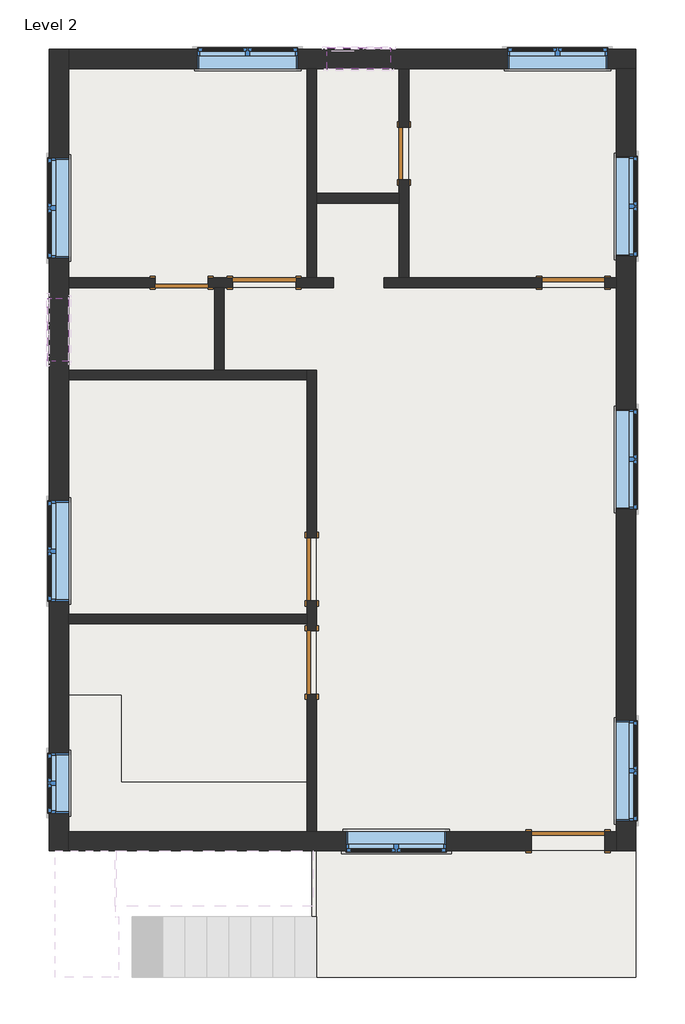
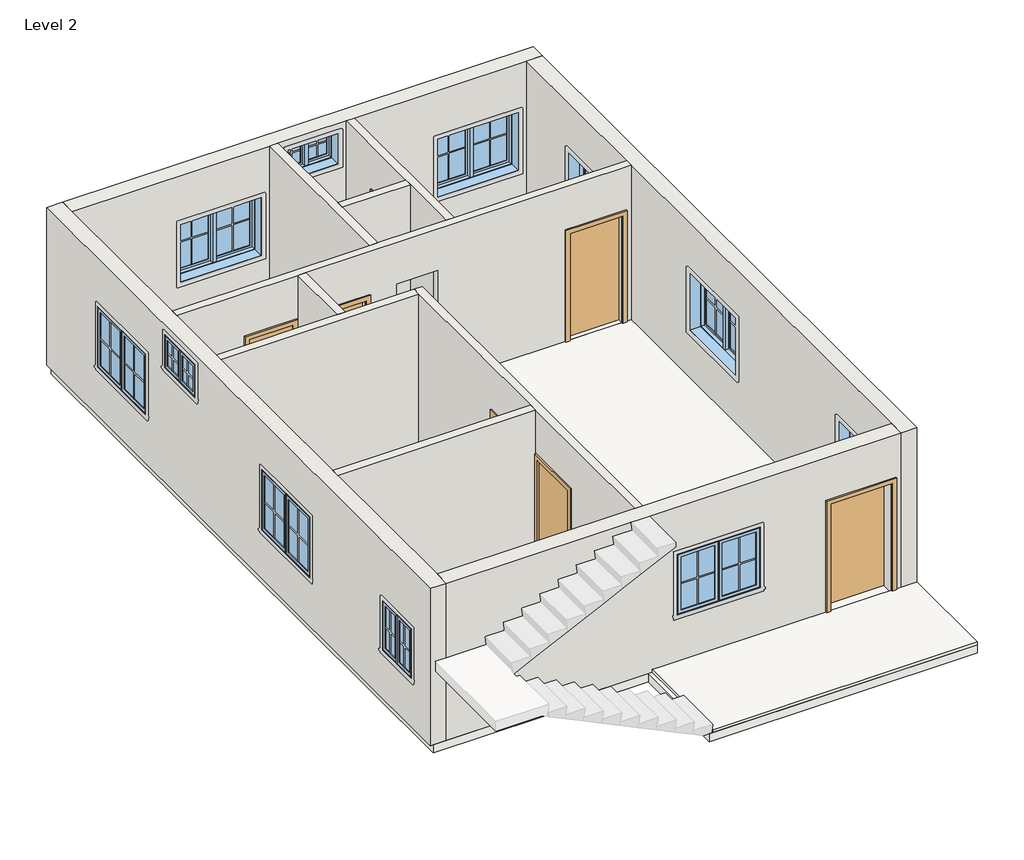
# One storey, part 1 of 2: 12 walls, 11 windows, 7 doors, 6 slabs.
"""IFC4 building model written with IfcOpenShell, lengths in millimetres."""

from ifc_helpers import new_model, si_unit, frame, origin, place, context, project, spatial, polyline, outline, extrude, faceted_brep, transform, mapped, element, save
from components import single_flush_3_6_472124c4, door_c78455d5, door_ad1ac78c, door_798417c2, window_casement_double_3_v2_9f1923e6, window_6eb120d7, window_2333f571

model = new_model("IFC4")

# Units and contexts
model_context = context("Model", 3, world=origin())
ifc_project = project(units=[si_unit("LENGTHUNIT", "METRE", prefix="MILLI")], contexts=[model_context])

# Site, building, storey
site = spatial("IfcSite", under=ifc_project)
building = spatial("IfcBuilding", under=site)
storey = spatial("IfcBuildingStorey", under=building, Name="Level 2", Elevation=3048.0)

# Doors
placement = place(None, origin())
single_flush_3_6_shape = single_flush_3_6_472124c4(model_context)
element("IfcDoor", 1, ObjectType="Single-Flush : 3'6", at=placement, inside=storey, context=model_context, shape_type="MappedRepresentation", body=[
    mapped(single_flush_3_6_shape, transform((-1353.6785282, -4927.3203663, 3048.0), x_axis=(1.0, 0.0, 0.0), y_axis=(0.0, 1.0, 0.0), z_axis=(0.0, 0.0, 1.0))),
])
door_shape = door_c78455d5(model_context)
element("IfcDoor", 2, ObjectType="Single-Flush : 30\" x 80\"", at=placement, inside=storey, context=model_context, shape_type="MappedRepresentation", body=[
    mapped(door_shape, transform((-6936.6570389, 3131.9303819, 3048.0), x_axis=(1.0, 0.0, 0.0), y_axis=(0.0, 1.0, 0.0), z_axis=(0.0, 0.0, 1.0))),
])
element("IfcDoor", 3, ObjectType="Single-Flush : 30\" x 80\"", at=placement, inside=storey, context=model_context, shape_type="MappedRepresentation", body=[
    mapped(door_shape, transform((-3724.1740631, 4999.2141951, 3048.0), x_axis=(0.0, -1.0, 0.0), y_axis=(1.0, 0.0, 0.0), z_axis=(0.0, 0.0, 1.0))),
])
door_2_shape = door_ad1ac78c(model_context)
element("IfcDoor", 4, ObjectType="Single-Flush : 36\" x 80\"", at=placement, inside=storey, context=model_context, shape_type="MappedRepresentation", body=[
    mapped(door_2_shape, transform((-5742.8570389, 3131.9303819, 3048.0), x_axis=(1.0, 0.0, 0.0), y_axis=(0.0, 1.0, 0.0), z_axis=(0.0, 0.0, 1.0))),
])
element("IfcDoor", 5, ObjectType="Single-Flush : 36\" x 80\"", at=placement, inside=storey, context=model_context, shape_type="MappedRepresentation", body=[
    mapped(door_2_shape, transform((-1277.4785282, 3131.9303819, 3048.0), x_axis=(1.0, 0.0, 0.0), y_axis=(0.0, 1.0, 0.0), z_axis=(0.0, 0.0, 1.0))),
])
element("IfcDoor", 6, ObjectType="Single-Flush : 36\" x 80\"", at=placement, inside=storey, context=model_context, shape_type="MappedRepresentation", body=[
    mapped(door_2_shape, transform((-5055.0449828, -2348.5368209, 3048.0), x_axis=(0.0, 1.0, 0.0), y_axis=(-1.0, 0.0, 0.0), z_axis=(0.0, 0.0, 1.0))),
])
door_3_shape = door_798417c2(model_context)
element("IfcDoor", 7, ObjectType="Single-Flush : 36\" x 80\"", at=placement, inside=storey, context=model_context, shape_type="MappedRepresentation", body=[
    mapped(door_3_shape, transform((-5055.0449828, -1002.3368209, 3048.0), x_axis=(0.0, -1.0, 0.0), y_axis=(1.0, 0.0, 0.0), z_axis=(0.0, 0.0, 1.0))),
])

# Slabs
element("IfcSlab", 8, ObjectType="6\"", at=placement, inside=storey, context=model_context, shape_type="SweptSolid", body=[
    extrude(outline(polyline([(-375.7785282, 6451.8796337), (-375.7785282, -6894.0922127), (-5049.0296925, -6894.0922127), (-5049.0296925, -5067.0203663), (-8797.003757, -5067.0203663), (-8797.003757, 6451.8796337), (-375.7785282, 6451.8796337)])), frame((0.0, 0.0, 2895.6), z_axis=(0.0, 0.0, 1.0), x_axis=(1.0, 0.0, 0.0)), (0.0, 0.0, 1.0), 152.4),
])
element("IfcSlab", 9, ObjectType="BED ROOM FLOOR", at=placement, inside=storey, context=model_context, shape_type="SweptSolid", body=[
    extrude(outline(polyline([(-4985.1949828, -4787.6203663), (-8569.7884077, -4787.6203663), (-8569.7884077, -1788.4748314), (-4985.1949828, -1788.4748314), (-4985.1949828, -4787.6203663)])), frame((0.0, 0.0, 3048.0), z_axis=(0.0, 0.0, 1.0), x_axis=(1.0, 0.0, 0.0)), (0.0, 0.0, 1.0), 50.8),
    extrude(outline(polyline([(-4985.1949828, -1672.5465885), (-8569.7884077, -1672.5465885), (-8569.7884077, 1731.1760727), (-4985.1949828, 1731.1760727), (-4985.1949828, -1672.5465885)])), frame((0.0, 0.0, 3048.0), z_axis=(0.0, 0.0, 1.0), x_axis=(1.0, 0.0, 0.0)), (0.0, 0.0, 1.0), 50.8),
    extrude(outline(polyline([(-8569.7884077, 6224.6642844), (-5124.8949828, 6224.6642844), (-5124.8949828, 3062.0803819), (-8569.7884077, 3062.0803819), (-8569.7884077, 6224.6642844)])), frame((0.0, 0.0, 3048.0), z_axis=(0.0, 0.0, 1.0), x_axis=(1.0, 0.0, 0.0)), (0.0, 0.0, 1.0), 50.8),
    extrude(outline(polyline([(-655.1785282, 6224.6642844), (-655.1785282, 3062.0803819), (-3654.3240631, 3062.0803819), (-3654.3240631, 6224.6642844), (-655.1785282, 6224.6642844)])), frame((0.0, 0.0, 3048.0), z_axis=(0.0, 0.0, 1.0), x_axis=(1.0, 0.0, 0.0)), (0.0, 0.0, 1.0), 50.8),
])
element("IfcSlab", 10, ObjectType="HALL FLOOR", at=placement, inside=storey, context=model_context, shape_type="SweptSolid", body=[
    extrude(outline(polyline([(-4985.1949828, -4787.6203663), (-4985.1949828, 1842.4631791), (-6320.7070389, 1842.4631791), (-6320.7070389, 3062.0803819), (-4744.7849815, 3062.0803819), (-4744.7849815, 3178.0086247), (-4985.1949828, 3178.0086247), (-4985.1949828, 4281.6641951), (-3765.6111695, 4281.6641951), (-3765.6111695, 3178.0086247), (-3997.4676553, 3178.0086247), (-3997.4676553, 3062.0803819), (-655.1785282, 3062.0803819), (-655.1785282, -4787.6203663), (-4985.1949828, -4787.6203663)])), frame((0.0, 0.0, 3048.0), z_axis=(0.0, 0.0, 1.0), x_axis=(1.0, 0.0, 0.0)), (0.0, 0.0, 1.0), 50.8),
])
element("IfcSlab", 11, ObjectType="HALL FLOOR", at=placement, inside=storey, context=model_context, shape_type="SweptSolid", body=[
    extrude(outline(polyline([(-375.7785282, -5067.0203663), (-375.7785282, -6894.0922127), (-4985.1949828, -6894.0922127), (-4985.1949828, -5067.0203663), (-375.7785282, -5067.0203663)])), frame((0.0, 0.0, 3048.0), z_axis=(0.0, 0.0, 1.0), x_axis=(1.0, 0.0, 0.0)), (0.0, 0.0, 1.0), 50.8),
])
element("IfcSlab", 12, ObjectType="KITCHEN BED", at=placement, inside=storey, context=model_context, shape_type="SweptSolid", body=[
    extrude(outline(polyline([(-7807.7884077, -2823.0618171), (-7807.7884077, -4077.7716275), (-5124.8949828, -4077.7716275), (-5124.8949828, -4839.7716275), (-7807.7884077, -4839.7716275), (-8569.7884077, -4839.7716275), (-8569.7884077, -2823.0618171), (-7807.7884077, -2823.0618171)])), frame((0.0, 0.0, 3860.8), z_axis=(0.0, 0.0, 1.0), x_axis=(1.0, 0.0, 0.0)), (0.0, 0.0, 1.0), 101.6),
])
element("IfcSlab", 13, ObjectType="TOILET FLOORING", at=placement, inside=storey, context=model_context, shape_type="SweptSolid", body=[
    extrude(outline(polyline([(-6432.0275348, 3201.7803819), (-6432.0275348, 1842.4631791), (-8569.7884077, 1842.4631791), (-8569.7884077, 3201.7803819), (-6432.0275348, 3201.7803819)])), frame((0.0, 0.0, 3048.0), z_axis=(0.0, 0.0, 1.0), x_axis=(1.0, 0.0, 0.0)), (0.0, 0.0, 1.0), 50.8),
    extrude(outline(polyline([(-3654.3240631, 6224.6642844), (-3654.3240631, 4397.592438), (-4985.1949828, 4397.592438), (-4985.1949828, 6224.6642844), (-3654.3240631, 6224.6642844)])), frame((0.0, 0.0, 3048.0), z_axis=(0.0, 0.0, 1.0), x_axis=(1.0, 0.0, 0.0)), (0.0, 0.0, 1.0), 50.8),
])

# Walls
element("IfcWall", 14, ObjectType="4.5\"", at=placement, inside=storey, context=model_context, shape_type="Brep", body=[
    faceted_brep([(-5124.8949828, -1459.5368209, 3048.0), (-5124.8949828, -1648.7748314, 3048.0), (-5124.8949828, -1788.4748314, 3048.0), (-5124.8949828, -1891.3368209, 3048.0), (-5124.8949828, -1891.3368209, 5080.0), (-5124.8949828, -2805.7368209, 5080.0), (-5124.8949828, -2805.7368209, 3048.0), (-5124.8949828, -4787.6203663, 3048.0), (-5124.8949828, -4787.6203663, 5943.6), (-5124.8949828, -1788.4748314, 5943.6), (-5124.8949828, -1648.7748314, 5943.6), (-5124.8949828, 1731.1760727, 5943.6), (-5124.8949828, 1870.8760727, 5943.6), (-5124.8949828, 1870.8760727, 3048.0), (-5124.8949828, 1731.1760727, 3048.0), (-5124.8949828, -545.1368209, 3048.0), (-5124.8949828, -545.1368209, 5080.0), (-5124.8949828, -1459.5368209, 5080.0), (-4985.1949828, -1891.3368209, 5080.0), (-4985.1949828, -1891.3368209, 3048.0), (-4985.1949828, -1459.5368209, 3048.0), (-4985.1949828, -1459.5368209, 5080.0), (-4985.1949828, -545.1368209, 5080.0), (-4985.1949828, -545.1368209, 3048.0), (-4985.1949828, 1870.8760727, 3048.0), (-4985.1949828, 1870.8760727, 5943.6), (-4985.1949828, -4787.6203663, 5943.6), (-4985.1949828, -4787.6203663, 3048.0), (-4985.1949828, -2805.7368209, 3048.0), (-4985.1949828, -2805.7368209, 5080.0)], [[[0, 1, 2, 3, 4, 5, 6, 7, 8, 9, 10, 11, 12, 13, 14, 15, 16, 17]], [[18, 19, 20, 21, 22, 23, 24, 25, 26, 27, 28, 29]], [[28, 27, 7, 6]], [[20, 19, 3, 2, 1, 0]], [[15, 14, 13, 24, 23]], [[12, 11, 10, 9, 8, 26, 25]], [[8, 7, 27, 26]], [[21, 20, 0, 17]], [[22, 21, 17, 16]], [[23, 22, 16, 15]], [[4, 3, 19, 18]], [[5, 4, 18, 29]], [[6, 5, 29, 28]], [[13, 12, 25, 24]]]),
])
element("IfcWall", 15, ObjectType="4.5\"", at=placement, inside=storey, context=model_context, shape_type="SweptSolid", body=[
    extrude(outline(polyline([(-8569.7884077, -1648.7748314), (-5124.8949828, -1648.7748314), (-5124.8949828, -1788.4748314), (-8569.7884077, -1788.4748314), (-8569.7884077, -1648.7748314)])), frame((0.0, 0.0, 3048.0), z_axis=(0.0, 0.0, 1.0), x_axis=(1.0, 0.0, 0.0)), (0.0, 0.0, 1.0), 2895.6),
])
element("IfcWall", 16, ObjectType="4.5\"", at=placement, inside=storey, context=model_context, shape_type="Brep", body=[
    faceted_brep([(-5124.8949828, 1870.8760727, 3048.0), (-6320.7070389, 1870.8760727, 3048.0), (-6460.4070389, 1870.8760727, 3048.0), (-8569.7884077, 1870.8760727, 3048.0), (-8569.7884077, 1870.8760727, 5943.6), (-6460.4070389, 1870.8760727, 5943.6), (-6320.7070389, 1870.8760727, 5943.6), (-5124.8949828, 1870.8760727, 5943.6), (-5124.8949828, 1731.1760727, 3048.0), (-5124.8949828, 1731.1760727, 5943.6), (-8569.7884077, 1731.1760727, 5943.6), (-8569.7884077, 1731.1760727, 3048.0)], [[[0, 1, 2, 3, 4, 5, 6, 7]], [[8, 9, 10, 11]], [[3, 2, 1, 0, 8, 11]], [[7, 6, 5, 4, 10, 9]], [[4, 3, 11, 10]], [[0, 7, 9, 8]]]),
])
element("IfcWall", 17, ObjectType="4.5\"", at=placement, inside=storey, context=model_context, shape_type="SweptSolid", body=[
    extrude(outline(polyline([(-6460.4070389, 1870.8760727), (-6460.4070389, 3062.0803819), (-6320.7070389, 3062.0803819), (-6320.7070389, 1870.8760727), (-6460.4070389, 1870.8760727)])), frame((0.0, 0.0, 3048.0), z_axis=(0.0, 0.0, 1.0), x_axis=(1.0, 0.0, 0.0)), (0.0, 0.0, 1.0), 2895.6),
])
element("IfcWall", 18, ObjectType="4.5\"", at=placement, inside=storey, context=model_context, shape_type="Brep", body=[
    faceted_brep([(-6200.0570389, 3201.7803819, 3048.0), (-6555.6570389, 3201.7803819, 3048.0), (-6555.6570389, 3201.7803819, 5080.0), (-7317.6570389, 3201.7803819, 5080.0), (-7317.6570389, 3201.7803819, 3048.0), (-8569.7884077, 3201.7803819, 3048.0), (-8569.7884077, 3201.7803819, 5943.6), (-5124.8949828, 3201.7803819, 5943.6), (-4985.1949828, 3201.7803819, 5943.6), (-3794.0240631, 3201.7803819, 5943.6), (-3654.3240631, 3201.7803819, 5943.6), (-655.1785282, 3201.7803819, 5943.6), (-655.1785282, 3201.7803819, 3048.0), (-820.2785282, 3201.7803819, 3048.0), (-820.2785282, 3201.7803819, 5080.0), (-1734.6785282, 3201.7803819, 5080.0), (-1734.6785282, 3201.7803819, 3048.0), (-3654.3240631, 3201.7803819, 3048.0), (-3794.0240631, 3201.7803819, 3048.0), (-4012.6375241, 3201.7803819, 3048.0), (-4012.6375241, 3201.7803819, 5181.6), (-4744.7849815, 3201.7803819, 5181.6), (-4744.7849815, 3201.7803819, 3048.0), (-4985.1949828, 3201.7803819, 3048.0), (-5124.8949828, 3201.7803819, 3048.0), (-5285.6570389, 3201.7803819, 3048.0), (-5285.6570389, 3201.7803819, 5080.0), (-6200.0570389, 3201.7803819, 5080.0), (-6555.6570389, 3062.0803819, 5080.0), (-6555.6570389, 3062.0803819, 3048.0), (-6460.4070389, 3062.0803819, 3048.0), (-6320.7070389, 3062.0803819, 3048.0), (-6200.0570389, 3062.0803819, 3048.0), (-6200.0570389, 3062.0803819, 5080.0), (-5285.6570389, 3062.0803819, 5080.0), (-5285.6570389, 3062.0803819, 3048.0), (-4744.7849815, 3062.0803819, 3048.0), (-4744.7849815, 3062.0803819, 5181.6), (-4012.6375241, 3062.0803819, 5181.6), (-4012.6375241, 3062.0803819, 3048.0), (-1734.6785282, 3062.0803819, 3048.0), (-1734.6785282, 3062.0803819, 5080.0), (-820.2785282, 3062.0803819, 5080.0), (-820.2785282, 3062.0803819, 3048.0), (-655.1785282, 3062.0803819, 3048.0), (-655.1785282, 3062.0803819, 5943.6), (-6320.7070389, 3062.0803819, 5943.6), (-6460.4070389, 3062.0803819, 5943.6), (-8569.7884077, 3062.0803819, 5943.6), (-8569.7884077, 3062.0803819, 3048.0), (-7317.6570389, 3062.0803819, 3048.0), (-7317.6570389, 3062.0803819, 5080.0)], [[[0, 1, 2, 3, 4, 5, 6, 7, 8, 9, 10, 11, 12, 13, 14, 15, 16, 17, 18, 19, 20, 21, 22, 23, 24, 25, 26, 27]], [[28, 29, 30, 31, 32, 33, 34, 35, 36, 37, 38, 39, 40, 41, 42, 43, 44, 45, 46, 47, 48, 49, 50, 51]], [[36, 35, 25, 24, 23, 22]], [[40, 39, 19, 18, 17, 16]], [[44, 43, 13, 12]], [[50, 49, 5, 4]], [[32, 31, 30, 29, 1, 0]], [[11, 10, 9, 8, 7, 6, 48, 47, 46, 45]], [[6, 5, 49, 48]], [[12, 11, 45, 44]], [[20, 38, 37, 21]], [[38, 20, 19, 39]], [[21, 37, 36, 22]], [[26, 25, 35, 34]], [[27, 26, 34, 33]], [[0, 27, 33, 32]], [[14, 13, 43, 42]], [[15, 14, 42, 41]], [[16, 15, 41, 40]], [[2, 1, 29, 28]], [[3, 2, 28, 51]], [[4, 3, 51, 50]]]),
])
element("IfcWall", 19, ObjectType="4.5\"", at=placement, inside=storey, context=model_context, shape_type="Brep", body=[
    faceted_brep([(-5124.8949828, 6224.6642844, 3048.0), (-5124.8949828, 3201.7803819, 3048.0), (-5124.8949828, 3201.7803819, 5943.6), (-5124.8949828, 6224.6642844, 5943.6), (-4985.1949828, 6224.6642844, 3048.0), (-4985.1949828, 6224.6642844, 5943.6), (-4985.1949828, 4421.3641951, 5943.6), (-4985.1949828, 4281.6641951, 5943.6), (-4985.1949828, 3201.7803819, 5943.6), (-4985.1949828, 3201.7803819, 3048.0), (-4985.1949828, 4281.6641951, 3048.0), (-4985.1949828, 4421.3641951, 3048.0)], [[[0, 1, 2, 3]], [[4, 5, 6, 7, 8, 9, 10, 11]], [[1, 0, 4, 11, 10, 9]], [[3, 2, 8, 7, 6, 5]], [[0, 3, 5, 4]], [[2, 1, 9, 8]]]),
])
element("IfcWall", 20, ObjectType="4.5\"", at=placement, inside=storey, context=model_context, shape_type="Brep", body=[
    faceted_brep([(-3794.0240631, 4618.2141951, 5080.0), (-3794.0240631, 4618.2141951, 3048.0), (-3794.0240631, 4421.3641951, 3048.0), (-3794.0240631, 4281.6641951, 3048.0), (-3794.0240631, 3201.7803819, 3048.0), (-3794.0240631, 3201.7803819, 5943.6), (-3794.0240631, 4281.6641951, 5943.6), (-3794.0240631, 4421.3641951, 5943.6), (-3794.0240631, 6224.6642844, 5943.6), (-3794.0240631, 6224.6642844, 3048.0), (-3794.0240631, 5380.2141951, 3048.0), (-3794.0240631, 5380.2141951, 5080.0), (-3654.3240631, 3201.7803819, 3048.0), (-3654.3240631, 4618.2141951, 3048.0), (-3654.3240631, 4618.2141951, 5080.0), (-3654.3240631, 5380.2141951, 5080.0), (-3654.3240631, 5380.2141951, 3048.0), (-3654.3240631, 6224.6642844, 3048.0), (-3654.3240631, 6224.6642844, 5943.6), (-3654.3240631, 3201.7803819, 5943.6)], [[[0, 1, 2, 3, 4, 5, 6, 7, 8, 9, 10, 11]], [[12, 13, 14, 15, 16, 17, 18, 19]], [[10, 9, 17, 16]], [[4, 3, 2, 1, 13, 12]], [[8, 7, 6, 5, 19, 18]], [[9, 8, 18, 17]], [[14, 13, 1, 0]], [[15, 14, 0, 11]], [[16, 15, 11, 10]], [[5, 4, 12, 19]]]),
])
element("IfcWall", 21, ObjectType="4.5\"", at=placement, inside=storey, context=model_context, shape_type="SweptSolid", body=[
    extrude(outline(polyline([(-4985.1949828, 4421.3641951), (-3794.0240631, 4421.3641951), (-3794.0240631, 4281.6641951), (-4985.1949828, 4281.6641951), (-4985.1949828, 4421.3641951)])), frame((0.0, 0.0, 3048.0), z_axis=(0.0, 0.0, 1.0), x_axis=(1.0, 0.0, 0.0)), (0.0, 0.0, 1.0), 2895.6),
])
element("IfcWall", 22, ObjectType="9\"", at=placement, inside=storey, context=model_context, shape_type="Brep", body=[
    faceted_brep([(-8849.1884077, 6504.0642844, 3048.0), (-8849.1884077, -5067.0203663, 3048.0), (-8849.1884077, -5067.0203663, 5943.6), (-8849.1884077, 6504.0642844, 5943.6), (-8849.1884077, -3657.3203663, 4876.8), (-8849.1884077, -4520.9203663, 4876.8), (-8849.1884077, -4520.9203663, 3962.4), (-8849.1884077, -3657.3203663, 3962.4), (-8849.1884077, 4935.3303819, 5080.0), (-8849.1884077, 3487.5303819, 5080.0), (-8849.1884077, 3487.5303819, 3962.4), (-8849.1884077, 4935.3303819, 3962.4), (-8849.1884077, -16.8248314, 5080.0), (-8849.1884077, -1464.6248314, 5080.0), (-8849.1884077, -1464.6248314, 3962.4), (-8849.1884077, -16.8248314, 3962.4), (-8849.1884077, 2910.9782273, 5791.2), (-8849.1884077, 1996.5782273, 5791.2), (-8849.1884077, 1996.5782273, 5181.6), (-8849.1884077, 2910.9782273, 5181.6), (-8569.7884077, 6504.0642844, 3048.0), (-8569.7884077, 6504.0642844, 5943.6), (-8569.7884077, 6224.6642844, 5943.6), (-8569.7884077, 3201.7803819, 5943.6), (-8569.7884077, 3062.0803819, 5943.6), (-8569.7884077, 1870.8760727, 5943.6), (-8569.7884077, 1731.1760727, 5943.6), (-8569.7884077, -1648.7748314, 5943.6), (-8569.7884077, -1788.4748314, 5943.6), (-8569.7884077, -4787.6203663, 5943.6), (-8569.7884077, -5067.0203663, 5943.6), (-8569.7884077, -5067.0203663, 3048.0), (-8569.7884077, -4787.6203663, 3048.0), (-8569.7884077, -1788.4748314, 3048.0), (-8569.7884077, -1648.7748314, 3048.0), (-8569.7884077, 1731.1760727, 3048.0), (-8569.7884077, 1870.8760727, 3048.0), (-8569.7884077, 3062.0803819, 3048.0), (-8569.7884077, 3201.7803819, 3048.0), (-8569.7884077, 6224.6642844, 3048.0), (-8569.7884077, -3657.3203663, 4876.8), (-8569.7884077, -3657.3203663, 3962.4), (-8569.7884077, -4520.9203663, 3962.4), (-8569.7884077, -4520.9203663, 4876.8), (-8569.7884077, 4935.3303819, 5080.0), (-8569.7884077, 4935.3303819, 3962.4), (-8569.7884077, 3487.5303819, 3962.4), (-8569.7884077, 3487.5303819, 5080.0), (-8569.7884077, -16.8248314, 5080.0), (-8569.7884077, -16.8248314, 3962.4), (-8569.7884077, -1464.6248314, 3962.4), (-8569.7884077, -1464.6248314, 5080.0), (-8569.7884077, 2910.9782273, 5791.2), (-8569.7884077, 2910.9782273, 5181.6), (-8569.7884077, 1996.5782273, 5181.6), (-8569.7884077, 1996.5782273, 5791.2)], [[[0, 1, 2, 3], [4, 5, 6, 7], [8, 9, 10, 11], [12, 13, 14, 15], [16, 17, 18, 19]], [[20, 21, 22, 23, 24, 25, 26, 27, 28, 29, 30, 31, 32, 33, 34, 35, 36, 37, 38, 39], [40, 41, 42, 43], [44, 45, 46, 47], [48, 49, 50, 51], [52, 53, 54, 55]], [[1, 0, 20, 39, 38, 37, 36, 35, 34, 33, 32, 31]], [[3, 2, 30, 29, 28, 27, 26, 25, 24, 23, 22, 21]], [[0, 3, 21, 20]], [[2, 1, 31, 30]], [[41, 40, 4, 7]], [[42, 41, 7, 6]], [[43, 42, 6, 5]], [[40, 43, 5, 4]], [[45, 44, 8, 11]], [[46, 45, 11, 10]], [[47, 46, 10, 9]], [[44, 47, 9, 8]], [[49, 48, 12, 15]], [[50, 49, 15, 14]], [[51, 50, 14, 13]], [[48, 51, 13, 12]], [[53, 52, 16, 19]], [[54, 53, 19, 18]], [[55, 54, 18, 17]], [[52, 55, 17, 16]]]),
])
element("IfcWall", 23, ObjectType="9\"", at=placement, inside=storey, context=model_context, shape_type="Brep", body=[
    faceted_brep([(-375.7785282, 6504.0642844, 3048.0), (-8569.7884077, 6504.0642844, 3048.0), (-8569.7884077, 6504.0642844, 5943.6), (-375.7785282, 6504.0642844, 5943.6), (-782.1785282, 6504.0642844, 5080.0), (-2229.9785282, 6504.0642844, 5080.0), (-2229.9785282, 6504.0642844, 3962.4), (-782.1785282, 6504.0642844, 3962.4), (-5258.2449828, 6504.0642844, 5080.0), (-6706.0449828, 6504.0642844, 5080.0), (-6706.0449828, 6504.0642844, 3962.4), (-5258.2449828, 6504.0642844, 3962.4), (-3919.7095229, 6504.0642844, 5791.2), (-4834.1095229, 6504.0642844, 5791.2), (-4834.1095229, 6504.0642844, 5181.6), (-3919.7095229, 6504.0642844, 5181.6), (-375.7785282, 6224.6642844, 3048.0), (-375.7785282, 6224.6642844, 5943.6), (-655.1785282, 6224.6642844, 5943.6), (-3654.3240631, 6224.6642844, 5943.6), (-3794.0240631, 6224.6642844, 5943.6), (-4985.1949828, 6224.6642844, 5943.6), (-5124.8949828, 6224.6642844, 5943.6), (-8569.7884077, 6224.6642844, 5943.6), (-8569.7884077, 6224.6642844, 3048.0), (-5124.8949828, 6224.6642844, 3048.0), (-4985.1949828, 6224.6642844, 3048.0), (-3794.0240631, 6224.6642844, 3048.0), (-3654.3240631, 6224.6642844, 3048.0), (-655.1785282, 6224.6642844, 3048.0), (-782.1785282, 6224.6642844, 5080.0), (-782.1785282, 6224.6642844, 3962.4), (-2229.9785282, 6224.6642844, 3962.4), (-2229.9785282, 6224.6642844, 5080.0), (-5258.2449828, 6224.6642844, 5080.0), (-5258.2449828, 6224.6642844, 3962.4), (-6706.0449828, 6224.6642844, 3962.4), (-6706.0449828, 6224.6642844, 5080.0), (-3919.7095229, 6224.6642844, 5791.2), (-3919.7095229, 6224.6642844, 5181.6), (-4834.1095229, 6224.6642844, 5181.6), (-4834.1095229, 6224.6642844, 5791.2)], [[[0, 1, 2, 3], [4, 5, 6, 7], [8, 9, 10, 11], [12, 13, 14, 15]], [[16, 17, 18, 19, 20, 21, 22, 23, 24, 25, 26, 27, 28, 29], [30, 31, 32, 33], [34, 35, 36, 37], [38, 39, 40, 41]], [[1, 0, 16, 29, 28, 27, 26, 25, 24]], [[3, 2, 23, 22, 21, 20, 19, 18, 17]], [[2, 1, 24, 23]], [[0, 3, 17, 16]], [[31, 30, 4, 7]], [[32, 31, 7, 6]], [[33, 32, 6, 5]], [[30, 33, 5, 4]], [[35, 34, 8, 11]], [[36, 35, 11, 10]], [[37, 36, 10, 9]], [[34, 37, 9, 8]], [[39, 38, 12, 15]], [[40, 39, 15, 14]], [[41, 40, 14, 13]], [[38, 41, 13, 12]]]),
])
element("IfcWall", 24, ObjectType="9\"", at=placement, inside=storey, context=model_context, shape_type="Brep", body=[
    faceted_brep([(-655.1785282, 6224.6642844, 3048.0), (-655.1785282, 3201.7803819, 3048.0), (-655.1785282, 3062.0803819, 3048.0), (-655.1785282, -4787.6203663, 3048.0), (-655.1785282, -5067.0203663, 3048.0), (-655.1785282, -5067.0203663, 5943.6), (-655.1785282, -4787.6203663, 5943.6), (-655.1785282, 3062.0803819, 5943.6), (-655.1785282, 3201.7803819, 5943.6), (-655.1785282, 6224.6642844, 5943.6), (-655.1785282, -4635.2203663, 5080.0), (-655.1785282, -4635.2203663, 3962.4), (-655.1785282, -3187.4203663, 3962.4), (-655.1785282, -3187.4203663, 5080.0), (-655.1785282, -139.4203663, 5080.0), (-655.1785282, -139.4203663, 3962.4), (-655.1785282, 1308.3796337, 3962.4), (-655.1785282, 1308.3796337, 5080.0), (-655.1785282, 3512.9303819, 5080.0), (-655.1785282, 3512.9303819, 3962.4), (-655.1785282, 4960.7303819, 3962.4), (-655.1785282, 4960.7303819, 5080.0), (-375.7785282, 6224.6642844, 3048.0), (-375.7785282, 6224.6642844, 5943.6), (-375.7785282, -5067.0203663, 5943.6), (-375.7785282, -5067.0203663, 3048.0), (-375.7785282, -4635.2203663, 5080.0), (-375.7785282, -3187.4203663, 5080.0), (-375.7785282, -3187.4203663, 3962.4), (-375.7785282, -4635.2203663, 3962.4), (-375.7785282, -139.4203663, 5080.0), (-375.7785282, 1308.3796337, 5080.0), (-375.7785282, 1308.3796337, 3962.4), (-375.7785282, -139.4203663, 3962.4), (-375.7785282, 3512.9303819, 5080.0), (-375.7785282, 4960.7303819, 5080.0), (-375.7785282, 4960.7303819, 3962.4), (-375.7785282, 3512.9303819, 3962.4)], [[[0, 1, 2, 3, 4, 5, 6, 7, 8, 9], [10, 11, 12, 13], [14, 15, 16, 17], [18, 19, 20, 21]], [[22, 23, 24, 25], [26, 27, 28, 29], [30, 31, 32, 33], [34, 35, 36, 37]], [[4, 3, 2, 1, 0, 22, 25]], [[9, 8, 7, 6, 5, 24, 23]], [[5, 4, 25, 24]], [[0, 9, 23, 22]], [[11, 10, 26, 29]], [[12, 11, 29, 28]], [[13, 12, 28, 27]], [[10, 13, 27, 26]], [[15, 14, 30, 33]], [[16, 15, 33, 32]], [[17, 16, 32, 31]], [[14, 17, 31, 30]], [[19, 18, 34, 37]], [[20, 19, 37, 36]], [[21, 20, 36, 35]], [[18, 21, 35, 34]]]),
])
element("IfcWall", 25, ObjectType="9\"", at=placement, inside=storey, context=model_context, shape_type="Brep", body=[
    faceted_brep([(-655.1785282, -4787.6203663, 3048.0), (-820.2785282, -4787.6203663, 3048.0), (-820.2785282, -4787.6203663, 5080.0), (-1887.0785282, -4787.6203663, 5080.0), (-1887.0785282, -4787.6203663, 3048.0), (-4985.1949828, -4787.6203663, 3048.0), (-5124.8949828, -4787.6203663, 3048.0), (-8569.7884077, -4787.6203663, 3048.0), (-8569.7884077, -4787.6203663, 5943.6), (-5124.8949828, -4787.6203663, 5943.6), (-4985.1949828, -4787.6203663, 5943.6), (-655.1785282, -4787.6203663, 5943.6), (-4559.7449828, -4787.6203663, 5080.0), (-4559.7449828, -4787.6203663, 3962.4), (-3111.9449828, -4787.6203663, 3962.4), (-3111.9449828, -4787.6203663, 5080.0), (-820.2785282, -5067.0203663, 5080.0), (-820.2785282, -5067.0203663, 3048.0), (-655.1785282, -5067.0203663, 3048.0), (-655.1785282, -5067.0203663, 5943.6), (-8569.7884077, -5067.0203663, 5943.6), (-8569.7884077, -5067.0203663, 3048.0), (-1887.0785282, -5067.0203663, 3048.0), (-1887.0785282, -5067.0203663, 5080.0), (-4559.7449828, -5067.0203663, 5080.0), (-3111.9449828, -5067.0203663, 5080.0), (-3111.9449828, -5067.0203663, 3962.4), (-4559.7449828, -5067.0203663, 3962.4)], [[[0, 1, 2, 3, 4, 5, 6, 7, 8, 9, 10, 11], [12, 13, 14, 15]], [[16, 17, 18, 19, 20, 21, 22, 23], [24, 25, 26, 27]], [[22, 21, 7, 6, 5, 4]], [[18, 17, 1, 0]], [[11, 10, 9, 8, 20, 19]], [[0, 11, 19, 18]], [[8, 7, 21, 20]], [[13, 12, 24, 27]], [[14, 13, 27, 26]], [[15, 14, 26, 25]], [[12, 15, 25, 24]], [[2, 1, 17, 16]], [[3, 2, 16, 23]], [[4, 3, 23, 22]]]),
])

# Windows
window_casement_double_3_v2_shape = window_casement_double_3_v2_9f1923e6(model_context)
element("IfcWindow", 26, ObjectType="Window-Casement-Double : 3'V2'", at=placement, inside=storey, context=model_context, shape_type="MappedRepresentation", body=[
    mapped(window_casement_double_3_v2_shape, transform((-8709.4884077, 2453.7782273, 4267.2), x_axis=(0.0, 1.0, 0.0), y_axis=(-1.0, 0.0, 0.0), z_axis=(0.0, 0.0, 1.0))),
])
element("IfcWindow", 27, ObjectType="Window-Casement-Double : 3'V2'", at=placement, inside=storey, context=model_context, shape_type="MappedRepresentation", body=[
    mapped(window_casement_double_3_v2_shape, transform((-4376.9095229, 6364.3642844, 4267.2), x_axis=(1.0, 0.0, 0.0), y_axis=(0.0, 1.0, 0.0), z_axis=(0.0, 0.0, 1.0))),
])
window_shape = window_6eb120d7(model_context)
element("IfcWindow", 28, ObjectType="Window-Casement-Double : 34\" x 36\"", at=placement, inside=storey, context=model_context, shape_type="MappedRepresentation", body=[
    mapped(window_shape, transform((-8709.4884077, -4089.1203663, 3048.0), x_axis=(0.0, 1.0, 0.0), y_axis=(-1.0, 0.0, 0.0), z_axis=(0.0, 0.0, 1.0))),
])
window_2_shape = window_2333f571(model_context)
element("IfcWindow", 29, ObjectType="Window-Casement-Double : 57\" x 44\"", at=placement, inside=storey, context=model_context, shape_type="MappedRepresentation", body=[
    mapped(window_2_shape, transform((-515.4785282, -3911.3203663, 3048.0), x_axis=(0.0, -1.0, 0.0), y_axis=(1.0, 0.0, 0.0), z_axis=(0.0, 0.0, 1.0))),
])
element("IfcWindow", 30, ObjectType="Window-Casement-Double : 57\" x 44\"", at=placement, inside=storey, context=model_context, shape_type="MappedRepresentation", body=[
    mapped(window_2_shape, transform((-515.4785282, 584.4796337, 3048.0), x_axis=(0.0, -1.0, 0.0), y_axis=(1.0, 0.0, 0.0), z_axis=(0.0, 0.0, 1.0))),
])
element("IfcWindow", 31, ObjectType="Window-Casement-Double : 57\" x 44\"", at=placement, inside=storey, context=model_context, shape_type="MappedRepresentation", body=[
    mapped(window_2_shape, transform((-515.4785282, 4236.8303819, 3048.0), x_axis=(0.0, -1.0, 0.0), y_axis=(1.0, 0.0, 0.0), z_axis=(0.0, 0.0, 1.0))),
])
element("IfcWindow", 32, ObjectType="Window-Casement-Double : 57\" x 44\"", at=placement, inside=storey, context=model_context, shape_type="MappedRepresentation", body=[
    mapped(window_2_shape, transform((-1506.0785282, 6364.3642844, 3048.0), x_axis=(1.0, 0.0, 0.0), y_axis=(0.0, 1.0, 0.0), z_axis=(0.0, 0.0, 1.0))),
])
element("IfcWindow", 33, ObjectType="Window-Casement-Double : 57\" x 44\"", at=placement, inside=storey, context=model_context, shape_type="MappedRepresentation", body=[
    mapped(window_2_shape, transform((-5982.1449828, 6364.3642844, 3048.0), x_axis=(1.0, 0.0, 0.0), y_axis=(0.0, 1.0, 0.0), z_axis=(0.0, 0.0, 1.0))),
])
element("IfcWindow", 34, ObjectType="Window-Casement-Double : 57\" x 44\"", at=placement, inside=storey, context=model_context, shape_type="MappedRepresentation", body=[
    mapped(window_2_shape, transform((-8709.4884077, 4211.4303819, 3048.0), x_axis=(0.0, 1.0, 0.0), y_axis=(-1.0, 0.0, 0.0), z_axis=(0.0, 0.0, 1.0))),
])
element("IfcWindow", 35, ObjectType="Window-Casement-Double : 57\" x 44\"", at=placement, inside=storey, context=model_context, shape_type="MappedRepresentation", body=[
    mapped(window_2_shape, transform((-8709.4884077, -740.7248314, 3048.0), x_axis=(0.0, 1.0, 0.0), y_axis=(-1.0, 0.0, 0.0), z_axis=(0.0, 0.0, 1.0))),
])
element("IfcWindow", 36, ObjectType="Window-Casement-Double : 57\" x 44\"", at=placement, inside=storey, context=model_context, shape_type="MappedRepresentation", body=[
    mapped(window_2_shape, transform((-3835.8449828, -4927.3203663, 3048.0), x_axis=(-1.0, 0.0, 0.0), y_axis=(0.0, -1.0, 0.0), z_axis=(0.0, 0.0, 1.0))),
])

save(model, "model.ifc")

# Revit data of these elements
# Type "Single-Flush : 3'6"
#   Type Mark = "8"
#   Construction Type Id = "MDOOR"
#   Assembly Code = "C1020"
#   Analytic Construction = "Metal"
#   Thickness = 2"
#   Heat Transfer Coefficient (U) = 0.651978 BTU/(h·ft²·°F)
#   Height = 80"
#   Trim Projection Ext = 1"
#   Trim Projection Int = 1"
#   Trim Width = 3"
#   Width = 42"
#   Define Thermal Properties by = 1
#   Door Material = Door - Panel
#   Frame Material = Door - Frame
#   Visual Light Transmittance = 0
#   Solar Heat Gain Coefficient = 0
#   Function = (empty or 0)
#   Wall Closure = (empty or 0)
# Type "Single-Flush : 30\" x 80\""
#   Type Mark = "5"
#   Construction Type Id = "MDOOR"
#   Assembly Code = "C1020"
#   Analytic Construction = "Metal"
#   Thickness = 2"
#   Heat Transfer Coefficient (U) = 0.651978 BTU/(h·ft²·°F)
#   Height = 80"
#   Trim Projection Ext = 1"
#   Trim Projection Int = 1"
#   Trim Width = 3"
#   Width = 30"
#   Define Thermal Properties by = 1
#   Define Thermal Properties by = 1
#   Door Material = Door - Panel
#   Frame Material = Door - Frame
#   Visual Light Transmittance = 0
#   Solar Heat Gain Coefficient = 0
#   Function = (empty or 0)
#   Wall Closure = (empty or 0)
# Type "Single-Flush : 36\" x 80\""
#   Type Mark = "6"
#   Construction Type Id = "MDOOR"
#   Assembly Code = "C1020"
#   Analytic Construction = "Metal"
#   Thickness = 2"
#   Heat Transfer Coefficient (U) = 0.651978 BTU/(h·ft²·°F)
#   Height = 80"
#   Trim Projection Ext = 1"
#   Trim Projection Int = 1"
#   Trim Width = 3"
#   Width = 36"
#   Define Thermal Properties by = 1
#   Define Thermal Properties by = 1
#   Door Material = Door - Panel
#   Frame Material = Door - Frame
#   Visual Light Transmittance = 0
#   Solar Heat Gain Coefficient = 0
#   Function = (empty or 0)
#   Wall Closure = (empty or 0)
# Type "6\""
#   Assembly Code = "B1010"
#   Function = 0
#   Layers, outside or top first: 6" no material (function 1)
# Type "BED ROOM FLOOR"
#   Assembly Code = "B1010"
#   Function = 0
#   Layers, outside or top first: 1" "BED ROOM FLOORING" (function 1); 1" no material (function 1)
# Type "HALL FLOOR"
#   Assembly Code = "B1010"
#   Function = 0
#   Layers, outside or top first: 1" "HALL FLOORING" (function 1); 1" no material (function 1)
# Type "KITCHEN BED"
#   Assembly Code = "B1010"
#   Function = 0
#   Layers, outside or top first: 1" "KITCHEN BED" (function 1); 3" no material (function 1)
# Type "TOILET FLOORING"
#   Assembly Code = "B1010"
#   Function = 0
#   Layers, outside or top first: 1" "TOILET FLOORING" (function 1); 1" no material (function 1)
# Type "4.5\""
#   Assembly Code = "B2010"
#   Layers, outside or top first: 0.5" "INNER WALL" (function 1); 4.5" "BRICK MATERIAL" (function 1); 0.5" "INNER WALL" (function 1)
# Type "9\""
#   Assembly Code = "B2010"
#   Layers, outside or top first: 1" "OUTER WALL" (function 4); 9" "BRICK MATERIAL" (function 1); 1" "OUTER WALL" (function 1)
# Type "Window-Casement-Double : 3'V2'"
#   Type Mark = "18"
#   Fire Rating = "0.5h"
#   Assembly Code = "B2020100"
#   Analytic Construction = "Double glazing - domestic"
#   Frame Extension [instance default] = 0.25"
#   Window Inset [instance default] = 0"
#   Wall Thickness [instance default] = 6"
#   Interior Wall Closure [instance default] = 2.25"
#   Half Width = 18"
#   Visual Light Transmittance = 0.81
#   Thermal Resistance (R) = 1.8146 (h·ft²·°F)/BTU
#   Solar Heat Gain Coefficient = 0.76
#   Rough Width = 36.5"
#   Rough Height = 24.5"
#   Height = 24"
#   Heat Transfer Coefficient (U) = 0.5511 BTU/(h·ft²·°F)
#   Exterior Wall Closure [instance default] = 1.25"
#   Extension Jamb [instance default] = 2.25"
#   Default Sill Height = 36"
#   Width = 36"
#   Muntin Visibility = yes
#   Interior Trim Visibility [instance default] = yes
#   Exterior Trim Visibility [instance default] = yes
#   Extension Jamb Visibility [instance default] = yes
#   Interior Trim Material = Wood - Stained
#   Muntin Pattern = Muntin Pattern_2x2 : Muntin Pattern_2x2
#   Interior Trim = Trim-Window-Interior-Flat : Picture Frame
#   Interior Frame Material = Wood - Stained
#   Glass Panel Material = Glass
#   Exterior Trim Material = Clad - White
#   Exterior Trim = Trim-Window-Exterior-Flat : with Sill
#   Exterior Frame Material = Clad - White
#   Wall Closure = (empty or 0)
# Type "Window-Casement-Double : 34\" x 36\""
#   Type Mark = "14"
#   Fire Rating = "0.5h"
#   Assembly Code = "B2020100"
#   Analytic Construction = "Double glazing - domestic"
#   Frame Extension [instance default] = 0.25"
#   Window Inset [instance default] = 0"
#   Wall Thickness [instance default] = 6"
#   Interior Wall Closure [instance default] = 2.25"
#   Half Width = 17"
#   Visual Light Transmittance = 0.81
#   Thermal Resistance (R) = 1.8146 (h·ft²·°F)/BTU
#   Solar Heat Gain Coefficient = 0.76
#   Rough Width = 34.5"
#   Rough Height = 36.5"
#   Height = 36"
#   Heat Transfer Coefficient (U) = 0.5511 BTU/(h·ft²·°F)
#   Exterior Wall Closure [instance default] = 1.25"
#   Extension Jamb [instance default] = 2.25"
#   Default Sill Height = 36"
#   Width = 34"
#   Define Thermal Properties by = 0
#   Muntin Visibility = yes
#   Interior Trim Visibility [instance default] = yes
#   Exterior Trim Visibility [instance default] = yes
#   Extension Jamb Visibility [instance default] = yes
#   Interior Trim Material = Wood - Stained
#   Muntin Pattern = Muntin Pattern_2x2 : Muntin Pattern_2x2
#   Interior Trim = Trim-Window-Interior-Flat : Picture Frame
#   Interior Frame Material = Wood - Stained
#   Glass Panel Material = Glass
#   Exterior Trim Material = Clad - White
#   Exterior Trim = Trim-Window-Exterior-Flat : with Sill
#   Exterior Frame Material = Clad - White
#   Wall Closure = (empty or 0)
# Type "Window-Casement-Double : 57\" x 44\""
#   Type Mark = "17"
#   Fire Rating = "0.5h"
#   Assembly Code = "B2020100"
#   Analytic Construction = "Double glazing - domestic"
#   Frame Extension [instance default] = 0.25"
#   Window Inset [instance default] = 0"
#   Wall Thickness [instance default] = 6"
#   Interior Wall Closure [instance default] = 2.25"
#   Half Width = 28.5"
#   Visual Light Transmittance = 0.81
#   Thermal Resistance (R) = 1.8146 (h·ft²·°F)/BTU
#   Solar Heat Gain Coefficient = 0.76
#   Rough Width = 57.5"
#   Rough Height = 44.5"
#   Height = 44"
#   Heat Transfer Coefficient (U) = 0.5511 BTU/(h·ft²·°F)
#   Exterior Wall Closure [instance default] = 1.25"
#   Extension Jamb [instance default] = 2.25"
#   Default Sill Height = 36"
#   Width = 57"
#   Define Thermal Properties by = 0
#   Muntin Visibility = yes
#   Interior Trim Visibility [instance default] = yes
#   Exterior Trim Visibility [instance default] = yes
#   Extension Jamb Visibility [instance default] = yes
#   Interior Trim Material = Wood - Stained
#   Muntin Pattern = Muntin Pattern_2x2 : Muntin Pattern_2x2
#   Interior Trim = Trim-Window-Interior-Flat : Picture Frame
#   Interior Frame Material = Wood - Stained
#   Glass Panel Material = Glass
#   Exterior Trim Material = Clad - White
#   Exterior Trim = Trim-Window-Exterior-Flat : with Sill
#   Exterior Frame Material = Clad - White
#   Wall Closure = (empty or 0)
# Element 1 (IfcDoor, "Single-Flush : 3'6")
#   Phase Created = New Construction
#   Materials on its faces: "Door - Frame", "Door - Panel"
# Elements 2, 3 (IfcDoor, "Single-Flush : 30\" x 80\"")
#   Phase Created = New Construction
#   Materials on its faces: "Door - Frame", "Door - Panel"
# Elements 4, 5, 6, 7 (IfcDoor, "Single-Flush : 36\" x 80\"")
#   Phase Created = New Construction
#   Materials on its faces: "Door - Frame", "Door - Panel"
# Element 8 (IfcSlab, "6\"")
#   Height Offset From Level = 0"
#   Phase Created = New Construction
#   Materials on its faces: "Default Floor"
# Element 9 (IfcSlab, "BED ROOM FLOOR")
#   built-in parameter 1001955 = -1.5708 (stored number, unit not read)
#   Height Offset From Level = 2"
#   Phase Created = New Construction
#   Materials on its faces: "Default Floor", "BED ROOM FLOORING"
# Element 10 (IfcSlab, "HALL FLOOR")
#   built-in parameter 1001955 = -1.5708 (stored number, unit not read)
#   Height Offset From Level = 2"
#   Phase Created = New Construction
#   Materials on its faces: "Default Floor", "HALL FLOORING"
# Element 11 (IfcSlab, "HALL FLOOR")
#   Height Offset From Level = 2"
#   Phase Created = New Construction
#   Materials on its faces: "Default Floor", "HALL FLOORING"
# Element 12 (IfcSlab, "KITCHEN BED")
#   Height Offset From Level = 36"
#   Phase Created = New Construction
#   Materials on its faces: "Default Floor", "KITCHEN BED"
# Element 13 (IfcSlab, "TOILET FLOORING")
#   Height Offset From Level = 2"
#   Phase Created = New Construction
#   Materials on its faces: "Default Floor", "TOILET FLOORING"
# Elements 14, 15, 16, 17, 18, 19, 20, 21 (IfcWall, "4.5\"")
#   Top Offset = 114"
#   Base Offset = 0"
#   wall height = 114"
#   Phase Created = New Construction
#   Base Constraint = Level 2
#   Top Constraint = Level 2
#   Materials on its faces: "Default Wall", "INNER WALL"
# Elements 22, 23, 24, 25 (IfcWall, "9\"")
#   Top Offset = 114"
#   Base Offset = 0"
#   wall height = 114"
#   Phase Created = New Construction
#   Base Constraint = Level 2
#   Top Constraint = Level 2
#   Materials on its faces: "Default Wall", "OUTER WALL"
# Element 26 (IfcWindow, "Window-Casement-Double : 3'V2'")
#   Mark = "20"
#   Window Inset = 0"
#   Interior Wall Closure = 2.25"
#   Frame Extension = 0.25"
#   Exterior Wall Closure = 1.25"
#   Interior Trim Visibility = yes
#   Exterior Trim Visibility = yes
#   Phase Created = New Construction
#   Materials on its faces: "Wood - Stained", "Glass", "Clad - White"
# Element 27 (IfcWindow, "Window-Casement-Double : 3'V2'")
#   Mark = "21"
#   Window Inset = 0"
#   Interior Wall Closure = 2.25"
#   Frame Extension = 0.25"
#   Exterior Wall Closure = 1.25"
#   Interior Trim Visibility = yes
#   Exterior Trim Visibility = yes
#   Phase Created = New Construction
#   Materials on its faces: "Wood - Stained", "Glass", "Clad - White"
# Element 28 (IfcWindow, "Window-Casement-Double : 34\" x 36\"")
#   Mark = "12"
#   Window Inset = 0"
#   Interior Wall Closure = 2.25"
#   Frame Extension = 0.25"
#   Exterior Wall Closure = 1.25"
#   Interior Trim Visibility = yes
#   Exterior Trim Visibility = yes
#   Phase Created = New Construction
#   Materials on its faces: "Wood - Stained", "Glass", "Clad - White"
# Element 29 (IfcWindow, "Window-Casement-Double : 57\" x 44\"")
#   Mark = "13"
#   Window Inset = 0"
#   Interior Wall Closure = 2.25"
#   Frame Extension = 0.25"
#   Exterior Wall Closure = 1.25"
#   Interior Trim Visibility = yes
#   Exterior Trim Visibility = yes
#   Phase Created = New Construction
#   Materials on its faces: "Wood - Stained", "Glass", "Clad - White"
# Element 30 (IfcWindow, "Window-Casement-Double : 57\" x 44\"")
#   Mark = "14"
#   Window Inset = 0"
#   Interior Wall Closure = 2.25"
#   Frame Extension = 0.25"
#   Exterior Wall Closure = 1.25"
#   Interior Trim Visibility = yes
#   Exterior Trim Visibility = yes
#   Phase Created = New Construction
#   Materials on its faces: "Wood - Stained", "Glass", "Clad - White"
# Element 31 (IfcWindow, "Window-Casement-Double : 57\" x 44\"")
#   Mark = "15"
#   Window Inset = 0"
#   Interior Wall Closure = 2.25"
#   Frame Extension = 0.25"
#   Exterior Wall Closure = 1.25"
#   Interior Trim Visibility = yes
#   Exterior Trim Visibility = yes
#   Phase Created = New Construction
#   Materials on its faces: "Wood - Stained", "Glass", "Clad - White"
# Element 32 (IfcWindow, "Window-Casement-Double : 57\" x 44\"")
#   Mark = "16"
#   Window Inset = 0"
#   Interior Wall Closure = 2.25"
#   Frame Extension = 0.25"
#   Exterior Wall Closure = 1.25"
#   Interior Trim Visibility = yes
#   Exterior Trim Visibility = yes
#   Phase Created = New Construction
#   Materials on its faces: "Wood - Stained", "Glass", "Clad - White"
# Element 33 (IfcWindow, "Window-Casement-Double : 57\" x 44\"")
#   Mark = "17"
#   Window Inset = 0"
#   Interior Wall Closure = 2.25"
#   Frame Extension = 0.25"
#   Exterior Wall Closure = 1.25"
#   Interior Trim Visibility = yes
#   Exterior Trim Visibility = yes
#   Phase Created = New Construction
#   Materials on its faces: "Wood - Stained", "Glass", "Clad - White"
# Element 34 (IfcWindow, "Window-Casement-Double : 57\" x 44\"")
#   Mark = "18"
#   Window Inset = 0"
#   Interior Wall Closure = 2.25"
#   Frame Extension = 0.25"
#   Exterior Wall Closure = 1.25"
#   Interior Trim Visibility = yes
#   Exterior Trim Visibility = yes
#   Phase Created = New Construction
#   Materials on its faces: "Wood - Stained", "Glass", "Clad - White"
# Element 35 (IfcWindow, "Window-Casement-Double : 57\" x 44\"")
#   Mark = "19"
#   Window Inset = 0"
#   Interior Wall Closure = 2.25"
#   Frame Extension = 0.25"
#   Exterior Wall Closure = 1.25"
#   Interior Trim Visibility = yes
#   Exterior Trim Visibility = yes
#   Phase Created = New Construction
#   Materials on its faces: "Wood - Stained", "Glass", "Clad - White"
# Element 36 (IfcWindow, "Window-Casement-Double : 57\" x 44\"")
#   Mark = "22"
#   Window Inset = 0"
#   Interior Wall Closure = 2.25"
#   Frame Extension = 0.25"
#   Exterior Wall Closure = 1.25"
#   Interior Trim Visibility = yes
#   Exterior Trim Visibility = yes
#   Phase Created = New Construction
#   Materials on its faces: "Wood - Stained", "Glass", "Clad - White"
# Materials
#   "Door - Panel": class "Wood", colour RGB 210 159 95, transparency 0, Cost = 0
#   "Door - Frame": colour RGB 118 70 51, transparency 0, Cost = 0
#   "BED ROOM FLOORING": class "Generic", colour RGB 65 88 108, transparency 0, Cost = 0
#   "HALL FLOORING": class "Generic", colour RGB 240 240 231, transparency 0, Cost = 0
#   "KITCHEN BED": class "Generic", colour RGB 193 98 95, transparency 0, Cost = 0
#   "TOILET FLOORING": class "Generic", colour RGB 206 206 206, transparency 0, Cost = 0
#   "INNER WALL": class "Generic", colour RGB 112 107 80, transparency 0, Cost = 0
#   "BRICK MATERIAL": class "Generic", colour RGB 86 33 38, transparency 0, Cost = 0
#   "OUTER WALL": class "Generic", colour RGB 231 231 228, transparency 0, Cost = 0
#   "Wood - Stained": class "Wood", colour RGB 224 178 126, transparency 0, Cost = 0
#   "Glass": class "Glass", colour RGB 0 128 192, transparency 0.75, Description = "Soda Lime Glass", Cost = 0
#   "Clad - White": class "Wood", colour RGB 242 242 238, transparency 0, Cost = 0
#   "Default Floor": colour RGB 128 128 128, transparency 0, Cost = 0
#   "Default Wall": colour RGB 128 128 128, transparency 0, Cost = 0
